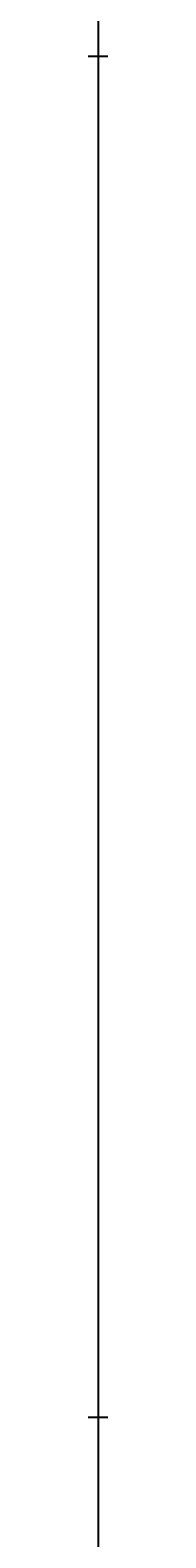
# Model space of a CAD drawing. Units: inches. Extents: x 35362 to 73946, y 43607 to 67532.
# Tile 29 of 134: x 48373 to 48373, y 46091 to 46564. Entities that reach past the tile are written whole.
import ezdxf

# ---------------------------------------------------------------- set-up
doc = ezdxf.new("R2010")
doc.units = ezdxf.units.IN
doc.header["$MEASUREMENT"] = 0
doc.layers.add('A-ANNO-DIMS', color=2, linetype='Continuous', lineweight=18)
doc.styles.get("Standard").update_dxf_attribs({"font": 'arial.ttf'})
doc.dimstyles.get("Standard").update_dxf_attribs({"dimtxt": 0.18, "dimasz": 0.18, "dimexe": 0.18, "dimexo": 0.0625, "dimgap": 0.09, "dimtad": 0, "dimtih": 1, "dimtoh": 1, "dimdec": 4, "dimzin": 0, "dimdsep": 46, "dimtxsty": 'Standard', "dimcen": 0.09, "dimadec": 0, "dimazin": 0, "dimtfac": 1, "dimtdec": 4, "dimtofl": 0, "dimtmove": 0, "dimatfit": 3, "dimfxl": 1, "dimtolj": 1, "dimtzin": 0, "dimarcsym": 0})

# ---------------------------------------------------------------- blocks, each defined once
blk = doc.blocks.new('*D5')
at = {"layer": 'A-ANNO-DIMS', "color": 0, "lineweight": -2, "transparency": 16777216}
for p, q in [((37121.95, 46919.32), (37121.95, 43606.68)), ((69871.5, 45449.83), (69871.5, 43606.68)), ((37122.13, 43606.86), (53496.29, 43606.86)), ((69871.32, 43606.86), (53497.15, 43606.86))]:
    blk.add_line(p, q, dxfattribs=at)
at = {"layer": 'A-ANNO-DIMS', "color": 0, "transparency": 16777216}
for points in [[(37122.13, 43606.89), (37122.13, 43606.83), (37121.95, 43606.86)], [(69871.32, 43606.89), (69871.32, 43606.83), (69871.5, 43606.86)]]:
    blk.add_solid(points, dxfattribs=at)
at = {"layer": 'Defpoints', "color": 0, "transparency": 16777216}
for p in [(37121.95, 46919.38), (69871.5, 45449.89), (69871.5, 43606.86)]:
    blk.add_point(p, dxfattribs=at)
at = {"layer": 'A-ANNO-DIMS', "color": 0, "transparency": 16777216, "insert": (53496.72, 43606.86), "char_height": 0.18, "attachment_point": 5}
blk.add_mtext('\\A1;32750', dxfattribs=at)
blk = doc.blocks.new('*D11')
at = {"layer": 'A-ANNO-DIMS', "color": 0, "lineweight": -2, "transparency": 16777216}
for p, q in [((47978.66, 56028.77), (47978.66, 43606.68)), ((53109.76, 56028.77), (53109.76, 43606.68)), ((47978.84, 43606.86), (50543.87, 43606.86)), ((53109.58, 43606.86), (50544.55, 43606.86))]:
    blk.add_line(p, q, dxfattribs=at)
at = {"layer": 'A-ANNO-DIMS', "color": 0, "transparency": 16777216}
for points in [[(47978.84, 43606.89), (47978.84, 43606.83), (47978.66, 43606.86)], [(53109.58, 43606.89), (53109.58, 43606.83), (53109.76, 43606.86)]]:
    blk.add_solid(points, dxfattribs=at)
at = {"layer": 'Defpoints', "color": 0, "transparency": 16777216}
for p in [(47978.66, 56028.84), (53109.76, 56028.84), (53109.76, 43606.86)]:
    blk.add_point(p, dxfattribs=at)
at = {"layer": 'A-ANNO-DIMS', "color": 0, "transparency": 16777216, "insert": (50544.21, 43606.86), "char_height": 0.18, "attachment_point": 5}
blk.add_mtext('\\A1;5131', dxfattribs=at)
blk = doc.blocks.new('*D27')
at = {"layer": 'A-ANNO-DIMS', "color": 0, "lineweight": -2, "transparency": 16777216}
for p, q in [((47978.66, 56028.77), (47978.66, 43606.68)), ((48373.49, 53428.96), (48373.49, 43606.68)), ((47978.84, 43606.86), (48175.68, 43606.86)), ((48373.31, 43606.86), (48176.47, 43606.86))]:
    blk.add_line(p, q, dxfattribs=at)
at = {"layer": 'A-ANNO-DIMS', "color": 0, "transparency": 16777216}
for points in [[(47978.84, 43606.89), (47978.84, 43606.83), (47978.66, 43606.86)], [(48373.31, 43606.89), (48373.31, 43606.83), (48373.49, 43606.86)]]:
    blk.add_solid(points, dxfattribs=at)
at = {"layer": 'Defpoints', "color": 0, "transparency": 16777216}
for p in [(47978.66, 56028.84), (48373.49, 53429.02), (48373.49, 43606.86)]:
    blk.add_point(p, dxfattribs=at)
at = {"layer": 'A-ANNO-DIMS', "color": 0, "transparency": 16777216, "insert": (48176.08, 43606.86), "char_height": 0.18, "attachment_point": 5}
blk.add_mtext('\\A1;394.8', dxfattribs=at)
blk = doc.blocks.new('*D67')
at = {"layer": 'A-ANNO-DIMS', "color": 0, "lineweight": -2, "transparency": 16777216}
for p, q in [((56873.54, 53351.53), (35361.77, 53351.53)), ((35361.95, 53351.35), (35361.95, 49400.89)), ((35361.95, 45450.07), (35361.95, 49400.53)), ((53793.58, 45449.89), (35361.77, 45449.89))]:
    blk.add_line(p, q, dxfattribs=at)
at = {"layer": 'A-ANNO-DIMS', "color": 0, "transparency": 16777216}
for points in [[(35361.92, 53351.35), (35361.98, 53351.35), (35361.95, 53351.53)], [(35361.92, 45450.07), (35361.98, 45450.07), (35361.95, 45449.89)]]:
    blk.add_solid(points, dxfattribs=at)
at = {"layer": 'Defpoints', "color": 0, "transparency": 16777216}
for p in [(35361.95, 53351.53), (56873.6, 53351.53), (53793.64, 45449.89)]:
    blk.add_point(p, dxfattribs=at)
at = {"layer": 'A-ANNO-DIMS', "color": 0, "transparency": 16777216, "insert": (35361.95, 49400.71), "char_height": 0.18, "attachment_point": 5}
blk.add_mtext('\\A1;7901.6', dxfattribs=at)
blk = doc.blocks.new('*D76')
at = {"layer": 'A-ANNO-DIMS', "color": 0, "lineweight": -2, "transparency": 16777216}
for p, q in [((54052.84, 46555.29), (35361.77, 46555.29)), ((35361.95, 46555.11), (35361.95, 46342.27)), ((35361.95, 46129.06), (35361.95, 46341.9)), ((53793.58, 46128.88), (35361.77, 46128.88))]:
    blk.add_line(p, q, dxfattribs=at)
at = {"layer": 'A-ANNO-DIMS', "color": 0, "transparency": 16777216}
for points in [[(35361.92, 46555.11), (35361.98, 46555.11), (35361.95, 46555.29)], [(35361.92, 46129.06), (35361.98, 46129.06), (35361.95, 46128.88)]]:
    blk.add_solid(points, dxfattribs=at)
at = {"layer": 'Defpoints', "color": 0, "transparency": 16777216}
for p in [(35361.95, 46555.29), (54052.9, 46555.29), (53793.64, 46128.88)]:
    blk.add_point(p, dxfattribs=at)
at = {"layer": 'A-ANNO-DIMS', "color": 0, "transparency": 16777216, "insert": (35361.95, 46342.09), "char_height": 0.18, "attachment_point": 5}
blk.add_mtext('\\A1;426.4', dxfattribs=at)
blk = doc.blocks.new('*D90')
at = {"layer": 'A-ANNO-DIMS', "color": 0, "lineweight": -2, "transparency": 16777216}
for p, q in [((53707.72, 47291.29), (35361.77, 47291.29)), ((35361.95, 47291.11), (35361.95, 46710.26)), ((35361.95, 46129.06), (35361.95, 46709.9)), ((53793.58, 46128.88), (35361.77, 46128.88))]:
    blk.add_line(p, q, dxfattribs=at)
at = {"layer": 'A-ANNO-DIMS', "color": 0, "transparency": 16777216}
for points in [[(35361.92, 47291.11), (35361.98, 47291.11), (35361.95, 47291.29)], [(35361.92, 46129.06), (35361.98, 46129.06), (35361.95, 46128.88)]]:
    blk.add_solid(points, dxfattribs=at)
at = {"layer": 'Defpoints', "color": 0, "transparency": 16777216}
for p in [(53707.78, 47291.29), (35361.95, 46128.88), (53793.64, 46128.88)]:
    blk.add_point(p, dxfattribs=at)
at = {"layer": 'A-ANNO-DIMS', "color": 0, "transparency": 16777216, "insert": (35361.95, 46710.08), "char_height": 0.18, "attachment_point": 5}
blk.add_mtext('\\A1;1162.4', dxfattribs=at)

msp = doc.modelspace()

# ---------------------------------------------------------------- dimensions: what is measured, and where the dimension line sits
at = {"layer": 'A-ANNO-DIMS'}
for base, p1, p2, override, picture, middle in [((53109.76, 43606.859), (47978.665, 56028.836), (53109.76, 56028.836), {"dimdec": 0, "dimlfac": 1, "dimrnd": 0, "dimzin": 0, "dimdsep": 46, "dimlunit": 2}, '*D11', (50544.212, 43606.859)), ((48373.492, 43606.859), (47978.665, 56028.836), (48373.492, 53429.019), {"dimdec": 1, "dimlfac": 1, "dimrnd": 0, "dimzin": 0, "dimdsep": 46, "dimlunit": 2}, '*D27', (48176.078, 43606.859)), ((69871.496, 43606.859), (37121.949, 46919.381), (69871.496, 45449.894), {"dimdec": 0, "dimlfac": 1, "dimrnd": 0, "dimzin": 0, "dimdsep": 46, "dimlunit": 2}, '*D5', (53496.723, 43606.859))]:
    dim = msp.add_linear_dim(base=base, p1=p1, p2=p2, dimstyle='Standard', override=override, dxfattribs=at)
    dim.commit()
    dim.dimension.update_dxf_attribs({"geometry": picture, "text_midpoint": middle})
for base, p1, p2, picture, middle in [((35361.949, 53351.529), (53793.638, 45449.894), (56873.602, 53351.529), '*D67', (35361.949, 49400.712)), ((35361.949, 46128.878), (53707.781, 47291.285), (53793.638, 46128.878), '*D90', (35361.949, 46710.081)), ((35361.949, 46555.293), (53793.638, 46128.878), (54052.899, 46555.293), '*D76', (35361.949, 46342.086))]:
    dim = msp.add_linear_dim(base=base, p1=p1, p2=p2, angle=90, dimstyle='Standard', override={"dimdec": 1, "dimlfac": 1, "dimrnd": 0, "dimzin": 0, "dimdsep": 46, "dimlunit": 2}, dxfattribs=at)
    dim.commit()
    dim.dimension.update_dxf_attribs({"geometry": picture, "text_midpoint": middle})

doc.saveas('drawing.dxf')
